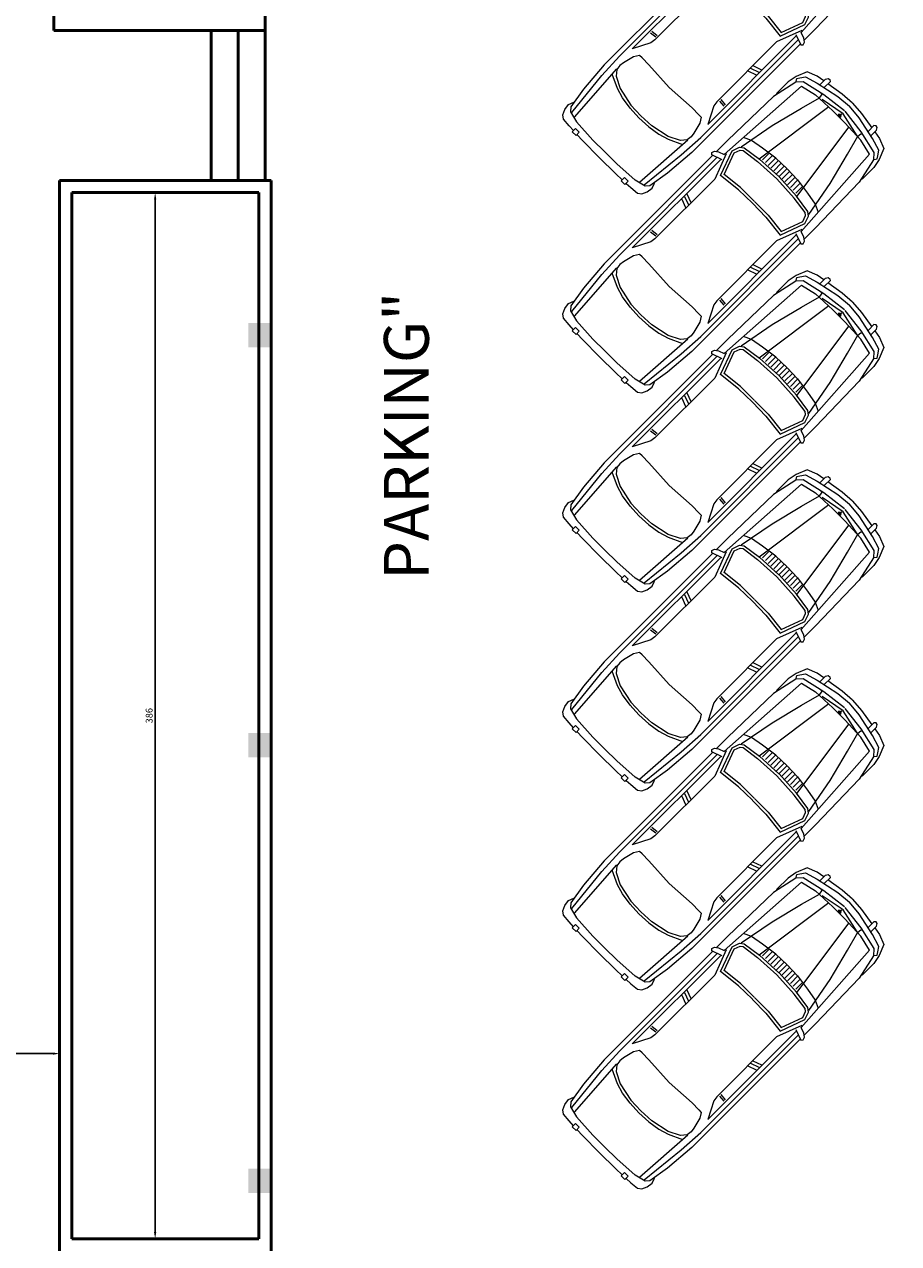
# Model space of a CAD drawing. Units: millimetres. Extents: x 2134 to 3363, y 1052 to 3233.
# Tile 7 of 11: x 2770 to 3093, y 2268 to 2718. Entities that reach past the tile are written whole.
import ezdxf

# ---------------------------------------------------------------- set-up
doc = ezdxf.new("R2010")
doc.units = ezdxf.units.MM
for name, color, linetype, lineweight in [('A-ANNO-DIMS', 2, 'Continuous', 18), ('A-AREA-IDEN', 3, 'Continuous', 18), ('A-COLS', 1, 'Continuous', 35), ('A-SITE-PRKG', 8, 'Continuous', 13), ('A-WALL', 7, 'Continuous', 50)]:
    doc.layers.add(name, color=color, linetype=linetype, lineweight=lineweight)
doc.styles.get("Standard").update_dxf_attribs({"font": 'arial.ttf'})
doc.styles.add('YQ_DIM', font='SUPEROS.SHX', dxfattribs={"width": 0.8, "bigfont": 'HZDX.SHX'})
doc.dimstyles.new('ISO-25', dxfattribs={"dimtxt": 2.5, "dimasz": 2.5, "dimexe": 1.25, "dimexo": 0.625, "dimtad": 1, "dimtxsty": 'Standard', "dimcen": 2.5, "dimadec": 0, "dimazin": 0, "dimtfac": 1, "dimtmove": 0, "dimatfit": 3, "dimfxl": 1, "dimarcsym": 0})

# ---------------------------------------------------------------- blocks, each defined once
blk = doc.blocks.new('A$C49703025')
for p, q in [((0.804, 0.813), (0.388, 0.78)), ((2.822, 0.813), (0.804, 0.813)), ((2.816, 0.829), (2.838, 0.849)), ((2.864, 0.684), (2.816, 0.829)), ((2.838, 0.849), (2.874, 0.835)), ((2.874, 0.835), (2.905, 0.791)), ((3.1, 0.813), (2.89, 0.813)), ((3.929, 0.795), (3.1, 0.813)), ((-0.089, 0.573), (-0.077, 0.686)), ((-0.077, 0.686), (-0.044, 0.735)), ((-0.044, 0.735), (0.024, 0.765)), ((0.057, 0.691), (0.02, 0.543)), ((0.024, 0.765), (0.105, 0.775)), ((0.881, 0.661), (0.04, 0.607)), ((0.105, 0.735), (0.057, 0.691)), ((0.061, 0.671), (0.683, 0.735)), ((0.388, 0.78), (0.105, 0.735)), ((0.105, 0.775), (0.174, 0.75)), ((0.683, 0.735), (1.027, 0.755)), ((0.707, 0.469), (0.792, 0.652)), ((0.877, 0.652), (0.808, 0.597)), ((0.942, 0.661), (0.877, 0.652)), ((1.002, 0.652), (0.942, 0.661)), ((1.152, 0.617), (1.002, 0.652)), ((1.027, 0.755), (2.841, 0.755)), ((1.443, 0.586), (1.212, 0.702)), ((1.212, 0.702), (2.85, 0.702)), ((1.538, 0.592), (1.529, 0.68)), ((1.566, 0.592), (1.557, 0.68)), ((2.125, 0.696), (2.083, 0.58)), ((2.174, 0.695), (2.132, 0.579)), ((2.219, 0.697), (2.178, 0.581)), ((2.958, 0.702), (2.618, 0.575)), ((2.707, 0.554), (3.041, 0.676)), ((2.905, 0.791), (2.932, 0.714)), ((2.932, 0.714), (4.286, 0.632)), ((3.041, 0.676), (3.144, 0.639)), ((3.317, 0.591), (3.271, 0.695)), ((4.269, 0.722), (3.929, 0.795)), ((3.993, 0.795), (3.965, 0.787)), ((4.2, 0.795), (3.993, 0.795)), ((4.328, 0.77), (4.2, 0.795)), ((4.343, 0.656), (4.269, 0.722)), ((4.279, 0.724), (4.312, 0.747)), ((4.312, 0.747), (4.35, 0.724)), ((4.472, 0.711), (4.328, 0.77)), ((4.412, 0.343), (4.343, 0.656)), ((4.35, 0.724), (4.407, 0.681)), ((4.407, 0.681), (4.461, 0.513)), ((4.525, 0.578), (4.472, 0.711)), ((-0.113, 0.489), (-0.053, 0.489)), ((-0.113, 0.42), (-0.113, 0.489)), ((-0.093, 0.489), (-0.089, 0.573)), ((-0.053, 0.489), (-0.053, 0.42)), ((0.02, 0.543), (0, 0.222)), ((0.808, 0.597), (0.732, 0.444)), ((1.217, 0.573), (1.152, 0.617)), ((1.221, 0.528), (1.217, 0.573)), ((1.221, 0.4), (1.221, 0.528)), ((1.507, 0.575), (1.443, 0.586)), ((2.618, 0.575), (1.507, 0.575)), ((2.741, 0.254), (2.707, 0.554)), ((2.747, 0.529), (3.041, 0.637)), ((2.778, 0.256), (2.747, 0.529)), ((3.041, 0.637), (3.122, 0.608)), ((3.122, 0.608), (3.148, 0.576)), ((3.144, 0.639), (3.183, 0.591)), ((3.148, 0.576), (3.18, 0.34)), ((3.163, 0.627), (3.648, 0.536)), ((3.183, 0.591), (3.217, 0.343)), ((3.35, 0.417), (3.317, 0.591)), ((3.648, 0.536), (4.083, 0.427)), ((4.286, 0.632), (4.337, 0.422)), ((4.461, 0.513), (4.529, 0.197)), ((4.542, 0.474), (4.525, 0.578)), ((-0.053, 0.42), (-0.113, 0.42)), ((-0.101, 0.306), (-0.096, 0.42)), ((0.643, 0.173), (0.667, 0.336)), ((0.667, 0.336), (0.707, 0.469)), ((0.732, 0.444), (0.679, 0.193)), ((1.196, 0), (1.221, 0.4)), ((3.18, 0.34), (3.198, 0)), ((3.217, 0.343), (3.235, 0.002)), ((3.22, 0.35), (4.35, 0.19)), ((3.38, 0.202), (3.35, 0.417)), ((4.083, 0.427), (4.344, 0.354)), ((4.337, 0.422), (4.348, 0.111)), ((4.344, 0.354), (4.395, 0.364)), ((4.395, 0.364), (4.404, 0.379)), ((4.456, 0.006), (4.412, 0.343)), ((4.473, 0.474), (4.574, 0.474)), ((4.592, 0.408), (4.49, 0.408)), ((4.59, 0.18), (4.553, 0.408)), ((4.574, 0.474), (4.606, 0.455)), ((4.609, 0.429), (4.592, 0.408)), ((4.606, 0.455), (4.609, 0.429)), ((-0.101, 0), (-0.101, 0.306)), ((0, 0.222), (0, 0)), ((0.635, 0), (0.643, 0.173)), ((0.679, 0.193), (0.671, 0)), ((2.744, 0.002), (2.741, 0.254)), ((2.781, 0.003), (2.778, 0.256)), ((3.241, 0.309), (3.365, 0.309)), ((3.241, 0.257), (3.373, 0.257)), ((3.241, 0.206), (3.382, 0.206)), ((3.386, 0.002), (3.38, 0.202)), ((4.415, -0.011), (4.354, 0.313)), ((4.529, 0.197), (4.546, -0.002)), ((4.599, 0), (4.59, 0.18)), ((-0.101, 0), (-0.101, -0.306)), ((0, -0.222), (0, 0)), ((0.635, 0), (0.643, -0.173)), ((0.679, -0.193), (0.671, 0)), ((1.196, 0), (1.221, -0.4)), ((3.241, 0.154), (3.382, 0.154)), ((3.241, 0.103), (3.382, 0.103)), ((3.241, 0.051), (3.382, 0.051)), ((3.241, 0), (3.382, 0)), ((4.348, 0.111), (4.348, -0.004)), ((4.348, -0.111), (4.348, 0.004)), ((4.363, 0.028), (4.359, 0.005)), ((4.359, 0.005), (4.363, -0.023)), ((4.386, 0.005), (4.363, 0.028)), ((4.529, -0.197), (4.546, 0.002)), ((4.599, 0), (4.59, -0.18)), ((2.744, -0.002), (2.741, -0.254)), ((2.781, -0.003), (2.778, -0.256)), ((3.18, -0.34), (3.198, 0)), ((3.217, -0.343), (3.235, -0.002)), ((3.241, -0.051), (3.382, -0.051)), ((3.241, -0.103), (3.382, -0.103)), ((3.241, -0.154), (3.382, -0.154)), ((3.386, -0.002), (3.38, -0.202)), ((4.337, -0.422), (4.348, -0.111)), ((4.344, -0.347), (4.415, -0.011)), ((4.401, 0), (4.354, 0)), ((4.363, -0.023), (4.382, -0.011)), ((4.456, -0.006), (4.412, -0.343)), ((-0.101, -0.306), (-0.096, -0.42)), ((0.02, -0.543), (0, -0.222)), ((0.643, -0.173), (0.667, -0.336)), ((0.732, -0.444), (0.679, -0.193)), ((2.741, -0.254), (2.707, -0.554)), ((2.778, -0.256), (2.747, -0.529)), ((3.22, -0.35), (4.35, -0.19)), ((3.241, -0.206), (3.382, -0.206)), ((3.241, -0.257), (3.373, -0.257)), ((3.241, -0.309), (3.365, -0.309)), ((3.38, -0.202), (3.35, -0.417)), ((4.461, -0.513), (4.529, -0.197)), ((4.59, -0.18), (4.553, -0.408)), ((-0.053, -0.42), (-0.113, -0.42)), ((-0.113, -0.42), (-0.113, -0.489)), ((-0.053, -0.489), (-0.053, -0.42)), ((0.667, -0.336), (0.707, -0.469)), ((0.707, -0.469), (0.792, -0.652)), ((0.808, -0.597), (0.732, -0.444)), ((1.221, -0.4), (1.221, -0.528)), ((3.148, -0.576), (3.18, -0.34)), ((3.183, -0.591), (3.217, -0.343)), ((3.35, -0.417), (3.317, -0.591)), ((3.648, -0.536), (4.083, -0.427)), ((4.083, -0.427), (4.344, -0.354)), ((4.286, -0.632), (4.337, -0.422)), ((4.412, -0.343), (4.343, -0.656)), ((4.344, -0.354), (4.395, -0.364)), ((4.395, -0.364), (4.404, -0.379)), ((4.473, -0.474), (4.574, -0.474)), ((4.592, -0.408), (4.49, -0.408)), ((4.542, -0.474), (4.525, -0.578)), ((4.574, -0.474), (4.606, -0.455)), ((4.609, -0.429), (4.592, -0.408)), ((4.606, -0.455), (4.609, -0.429)), ((-0.113, -0.489), (-0.053, -0.489)), ((-0.093, -0.489), (-0.089, -0.573)), ((-0.089, -0.573), (-0.077, -0.686)), ((0.057, -0.691), (0.02, -0.543)), ((0.881, -0.661), (0.04, -0.607)), ((0.877, -0.652), (0.808, -0.597)), ((1.152, -0.617), (1.002, -0.652)), ((1.217, -0.573), (1.152, -0.617)), ((1.443, -0.586), (1.212, -0.702)), ((1.221, -0.528), (1.217, -0.573)), ((1.507, -0.575), (1.443, -0.586)), ((2.618, -0.575), (1.507, -0.575)), ((1.538, -0.592), (1.529, -0.68)), ((1.566, -0.592), (1.557, -0.68)), ((2.125, -0.696), (2.083, -0.58)), ((2.174, -0.695), (2.132, -0.579)), ((2.219, -0.697), (2.178, -0.581)), ((2.958, -0.702), (2.618, -0.575)), ((2.707, -0.554), (3.041, -0.676)), ((2.747, -0.529), (3.041, -0.637)), ((2.932, -0.714), (4.286, -0.632)), ((3.041, -0.637), (3.122, -0.608)), ((3.041, -0.676), (3.144, -0.639)), ((3.122, -0.608), (3.148, -0.576)), ((3.144, -0.639), (3.183, -0.591)), ((3.163, -0.627), (3.648, -0.536)), ((3.317, -0.591), (3.271, -0.695)), ((4.407, -0.681), (4.461, -0.513)), ((4.525, -0.578), (4.472, -0.711)), ((-0.077, -0.686), (-0.044, -0.735)), ((-0.044, -0.735), (0.024, -0.765)), ((0.024, -0.765), (0.105, -0.775)), ((0.105, -0.735), (0.057, -0.691)), ((0.061, -0.671), (0.683, -0.735)), ((0.388, -0.78), (0.105, -0.735)), ((0.105, -0.775), (0.174, -0.75)), ((0.804, -0.813), (0.388, -0.78)), ((0.683, -0.735), (1.027, -0.755)), ((0.942, -0.661), (0.877, -0.652)), ((1.002, -0.652), (0.942, -0.661)), ((1.027, -0.755), (2.841, -0.755)), ((1.212, -0.702), (2.85, -0.702)), ((2.864, -0.684), (2.816, -0.829)), ((2.874, -0.835), (2.905, -0.791)), ((2.905, -0.791), (2.932, -0.714)), ((3.929, -0.795), (3.1, -0.813)), ((4.269, -0.722), (3.929, -0.795)), ((3.993, -0.795), (3.965, -0.787)), ((4.2, -0.795), (3.993, -0.795)), ((4.328, -0.77), (4.2, -0.795)), ((4.343, -0.656), (4.269, -0.722)), ((4.279, -0.724), (4.312, -0.747)), ((4.312, -0.747), (4.35, -0.724)), ((4.472, -0.711), (4.328, -0.77)), ((4.35, -0.724), (4.407, -0.681)), ((2.822, -0.813), (0.804, -0.813)), ((2.816, -0.829), (2.838, -0.849)), ((2.838, -0.849), (2.874, -0.835)), ((3.1, -0.813), (2.89, -0.813))]:
    blk.add_line(p, q)
blk = doc.blocks.new('*D11')
at = {"layer": 'A-ANNO-DIMS', "color": 0, "lineweight": -2, "transparency": 16777216}
for p, q in [((2821.78, 2655.46), (2817.4, 2655.46)), ((2818.65, 2652.96), (2818.65, 2271.96)), ((2821.78, 2269.46), (2817.4, 2269.46))]:
    blk.add_line(p, q, dxfattribs=at)
at = {"layer": 'A-ANNO-DIMS', "color": 0, "transparency": 16777216}
for points in [[(2818.23, 2652.96), (2819.06, 2652.96), (2818.65, 2655.46)], [(2818.23, 2271.96), (2819.06, 2271.96), (2818.65, 2269.46)]]:
    blk.add_solid(points, dxfattribs=at)
at = {"layer": 'Defpoints', "color": 0, "transparency": 16777216}
for p in [(2822.4, 2655.46), (2818.65, 2269.46), (2822.4, 2269.46)]:
    blk.add_point(p, dxfattribs=at)
at = {"layer": 'A-ANNO-DIMS', "color": 0, "transparency": 16777216, "insert": (2816.75, 2462.46), "char_height": 2.5, "attachment_point": 5, "rotation": 90}
blk.add_mtext('386', dxfattribs=at)
blk = doc.blocks.new('*D12')
at = {"layer": 'A-ANNO-DIMS', "color": 0, "lineweight": -2, "transparency": 16777216}
for p, q in [((2733.28, 2333.03), (2733.28, 2339.03)), ((2735.78, 2337.78), (2780.9, 2337.78)), ((2783.4, 2333.03), (2783.4, 2339.03))]:
    blk.add_line(p, q, dxfattribs=at)
at = {"layer": 'A-ANNO-DIMS', "color": 0, "transparency": 16777216}
for points in [[(2735.78, 2338.2), (2735.78, 2337.36), (2733.28, 2337.78)], [(2780.9, 2338.2), (2780.9, 2337.36), (2783.4, 2337.78)]]:
    blk.add_solid(points, dxfattribs=at)
at = {"layer": 'Defpoints', "color": 0, "transparency": 16777216}
for p in [(2783.4, 2337.78), (2733.28, 2332.41), (2783.4, 2332.41)]:
    blk.add_point(p, dxfattribs=at)
at = {"layer": 'A-ANNO-DIMS', "color": 0, "transparency": 16777216, "insert": (2758.34, 2339.91), "char_height": 2.5, "attachment_point": 5}
blk.add_mtext('50,12', dxfattribs=at)

msp = doc.modelspace()

# ---------------------------------------------------------------- hatches: boundary and pattern name
at = {"layer": 'A-COLS'}
h = msp.add_hatch(color=256, dxfattribs=at)
h.dxf.hatch_style = 1
h.paths.add_polyline_path([(2861.978, 2607.375), (2852.978, 2607.375), (2852.978, 2598.375), (2861.978, 2598.375)])
h = msp.add_hatch(color=256, dxfattribs=at)
h.dxf.hatch_style = 1
h.paths.add_polyline_path([(2861.978, 2456.066), (2852.978, 2456.066), (2852.978, 2447.066), (2861.978, 2447.066)])
h = msp.add_hatch(color=256, dxfattribs=at)
h.dxf.hatch_style = 1
h.paths.add_polyline_path([(2861.978, 2295.375), (2852.978, 2295.375), (2852.978, 2286.375), (2861.978, 2286.375)])

# ---------------------------------------------------------------- linework, layer by layer
at = {"layer": 'A-WALL'}
for p, q in [((2781.282, 3012.274), (2781.282, 2715.274)), ((2859.282, 3012.274), (2859.282, 2715.274)), ((2781.282, 2715.274), (2859.282, 2715.274)), ((2849.282, 2715.274), (2839.282, 2715.274)), ((2839.282, 2715.274), (2839.282, 2659.962)), ((2849.282, 2659.962), (2849.282, 2715.274)), ((2859.282, 2715.274), (2859.282, 2659.962)), ((2783.402, 2659.962), (2861.402, 2659.962)), ((2783.402, 2659.962), (2783.402, 2264.962)), ((2859.282, 2659.962), (2849.282, 2659.962)), ((2861.402, 2659.962), (2861.402, 2264.962)), ((2787.902, 2655.462), (2856.902, 2655.462)), ((2787.902, 2655.462), (2787.902, 2269.462)), ((2856.902, 2655.462), (2856.902, 2269.462)), ((2787.902, 2269.462), (2856.902, 2269.462))]:
    msp.add_line(p, q, dxfattribs=at)

# ---------------------------------------------------------------- block references
at = {"layer": 'A-SITE-PRKG', "xscale": 28.10227870703558, "yscale": 28.10227870703558, "zscale": 28.10227870703558, "rotation": 45}
for p in [(2984.561, 2670.442), (2984.561, 2597.017), (2984.561, 2523.591), (2984.561, 2450.165), (2984.561, 2376.739), (2984.561, 2303.313)]:
    msp.add_blockref('A$C49703025', p, dxfattribs=at)

# ---------------------------------------------------------------- texts
at = {"layer": 'A-AREA-IDEN', "insert": (2903.072, 2512.584), "char_height": 16.56819, "attachment_point": 1, "rotation": 90, "style": 'YQ_DIM'}
msp.add_mtext_dynamic_manual_height_columns('{\\f@FZYaoTi|b0|i0|c134|p2;PARKING"}', width=128.94034, gutter_width=26.518, heights=[0], dxfattribs=at)

# ---------------------------------------------------------------- dimensions: what is measured, and where the dimension line sits
at = {"layer": 'A-ANNO-DIMS'}
dim = msp.add_linear_dim(base=(2818.647, 2269.462), p1=(2822.402, 2655.462), p2=(2822.402, 2269.462), angle=90, dimstyle='ISO-25', override={"dimclrd": 0, "dimclre": 0, "dimclrt": 0}, dxfattribs=at)
dim.commit()
dim.dimension.update_dxf_attribs({"geometry": '*D11', "text_midpoint": (2816.745, 2462.462)})
dim = msp.add_linear_dim(base=(2783.402, 2337.781), p1=(2733.282, 2332.407), p2=(2783.402, 2332.407), dimstyle='ISO-25', override={"dimclrd": 0, "dimclre": 0, "dimclrt": 0}, dxfattribs=at)
dim.commit()
dim.dimension.update_dxf_attribs({"geometry": '*D12', "text_midpoint": (2758.342, 2339.909)})

doc.saveas('drawing.dxf')
